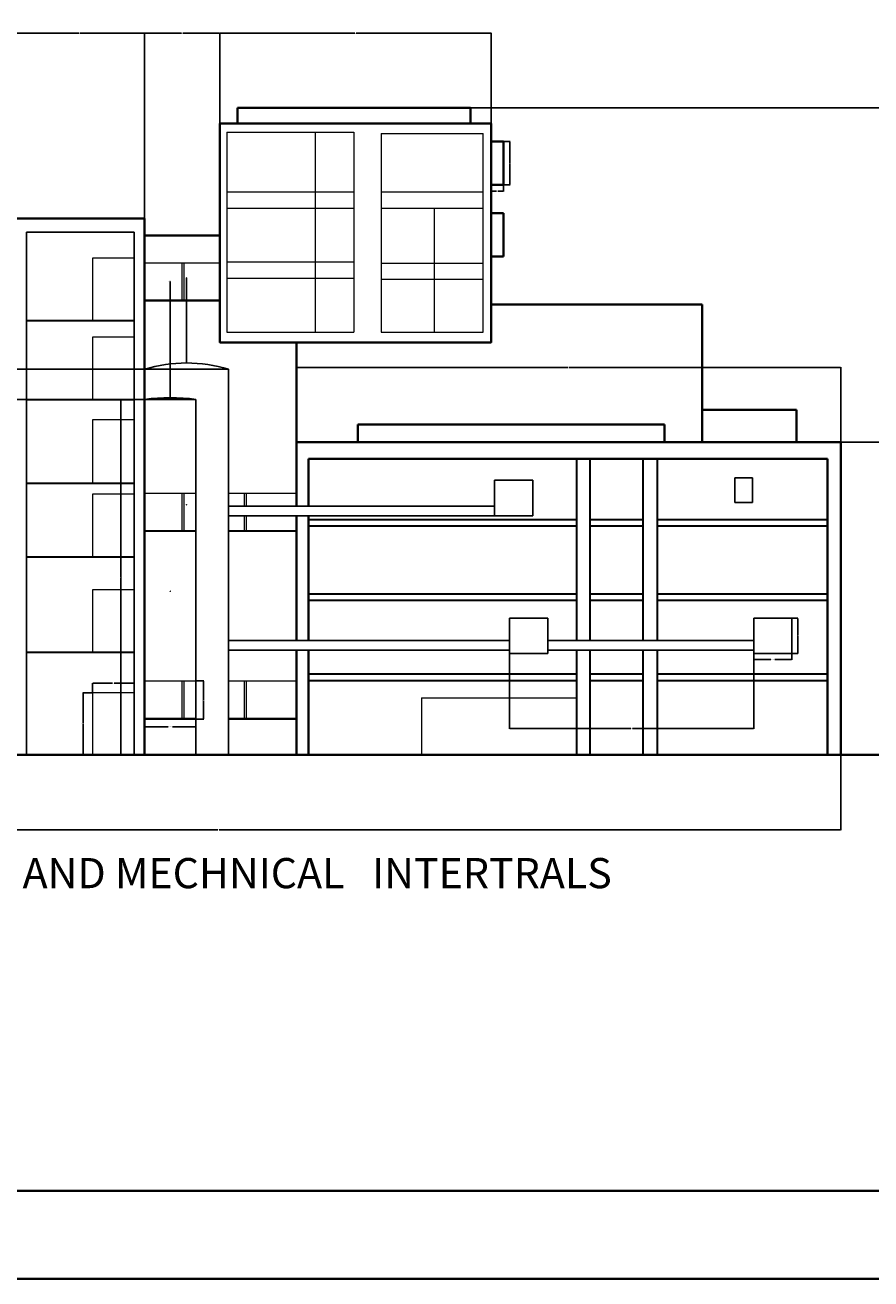
# Model space of a CAD drawing. Units: inches. Extents: x -934 to 898, y -1502 to 444.
# Tile 3 of 10: x -246 to 268, y -1502 to -739. Entities that reach past the tile are written whole.
import ezdxf

# ---------------------------------------------------------------- set-up
doc = ezdxf.new("R2010")
doc.units = ezdxf.units.IN
doc.header["$MEASUREMENT"] = 0
for name, color, linetype, lineweight in [('A-ANNO-DIMS', 2, 'Continuous', 18), ('A-ANNO-TITL', 7, 'Continuous', 30), ('A-ANNO-TTLB', 7, 'Continuous', 35), ('A-COLS', 1, 'Continuous', 30), ('A-DOOR', 3, 'Continuous', 18), ('A-ELEV', 7, 'Continuous', 35), ('A-FLOR', 7, 'Continuous', 30), ('A-GLAZ', 4, 'Continuous', 13), ('A-ROOF', 7, 'Continuous', 35), ('L-GRND', 7, 'Continuous', 35), ('M-HVAC', 6, 'Continuous', 25)]:
    doc.layers.add(name, color=color, linetype=linetype, lineweight=lineweight)
doc.styles.get("Standard").update_dxf_attribs({"font": 'arial.ttf'})
doc.dimstyles.get("Standard").update_dxf_attribs({"dimtxt": 0.18, "dimasz": 0.18, "dimexe": 0.18, "dimexo": 0.0625, "dimgap": 0.09, "dimtad": 0, "dimtih": 1, "dimtoh": 1, "dimdec": 4, "dimzin": 0, "dimdsep": 46, "dimtxsty": 'Standard', "dimcen": 0.09, "dimadec": 0, "dimazin": 0, "dimtfac": 1, "dimtdec": 4, "dimtofl": 0, "dimtmove": 0, "dimatfit": 3, "dimfxl": 1, "dimtolj": 1, "dimtzin": 0, "dimarcsym": 0})

# ---------------------------------------------------------------- blocks, each defined once
blk = doc.blocks.new('CORE-ACCESS-OPENING')
for p, q in [((25.27, 37.91), (0, 37.91)), ((0, 37.91), (0, 0))]:
    blk.add_line(p, q)
blk = doc.blocks.new('FACADE-PROJECTION-SHORT')
for p, q in [((0, 26.24), (7.46, 26.24)), ((7.46, 26.24), (7.46, 0)), ((7.46, 0), (0, 0))]:
    blk.add_line(p, q)
blk = doc.blocks.new('MECH-TERMINAL')
for p, q in [((0, 15.62), (0, 21.53)), ((0, 21.53), (23.24, 21.53)), ((0, 15.62), (0, 21.53)), ((0, 21.53), (23.24, 21.53)), ((0, 0), (0, 15.62)), ((0, 0), (0, 15.62)), ((23.24, 21.53), (23.24, 0)), ((23.24, 21.53), (23.24, 0)), ((23.24, 0), (0, 0)), ((23.24, 0), (0, 0))]:
    blk.add_line(p, q)
blk = doc.blocks.new('SHAFT-CONNECTOR-BAY')
for p, q in [((0, 23.2), (31.08, 23.2)), ((22.68, 23.2), (22.68, 0)), ((23.92, 23.2), (23.92, 0)), ((0, 0.56), (31.08, 0.56)), ((23.92, 0.56), (31.08, 0.56)), ((0, 0), (31.08, 0)), ((23.92, 0), (31.08, 0))]:
    blk.add_line(p, q)
blk = doc.blocks.new('*D67')
at = {"layer": 'A-ANNO-DIMS', "color": 0, "lineweight": -2, "transparency": 16777216}
for p, q in [((-204.98, -1145.23), (-210.79, -1145.23)), ((-210.61, -1145.41), (-210.61, -1164)), ((-210.61, -1182.96), (-210.61, -1164.37)), ((-204.98, -1183.14), (-210.79, -1183.14))]:
    blk.add_line(p, q, dxfattribs=at)
at = {"layer": 'A-ANNO-DIMS', "color": 0, "transparency": 16777216}
for points in [[(-210.64, -1145.41), (-210.58, -1145.41), (-210.61, -1145.23)], [(-210.64, -1182.96), (-210.58, -1182.96), (-210.61, -1183.14)]]:
    blk.add_solid(points, dxfattribs=at)
at = {"layer": 'Defpoints', "color": 0, "transparency": 16777216}
for p in [(-210.61, -1145.23), (-204.92, -1145.23), (-204.92, -1183.14)]:
    blk.add_point(p, dxfattribs=at)
at = {"layer": 'A-ANNO-DIMS', "color": 0, "transparency": 16777216, "insert": (-210.61, -1164.18), "char_height": 0.18, "attachment_point": 5}
blk.add_mtext('\\A1;ACCESS 38 TYP.', dxfattribs=at)
blk = doc.blocks.new('*D68')
at = {"layer": 'A-ANNO-DIMS', "color": 0, "lineweight": -2, "transparency": 16777216}
for p, q in [((-204.92, -1145.17), (-204.92, -1139.36)), ((-204.74, -1139.54), (-192.82, -1139.54)), ((-179.83, -1139.54), (-191.76, -1139.54)), ((-179.65, -1145.17), (-179.65, -1139.36))]:
    blk.add_line(p, q, dxfattribs=at)
at = {"layer": 'A-ANNO-DIMS', "color": 0, "transparency": 16777216}
for points in [[(-204.74, -1139.51), (-204.74, -1139.57), (-204.92, -1139.54)], [(-179.83, -1139.51), (-179.83, -1139.57), (-179.65, -1139.54)]]:
    blk.add_solid(points, dxfattribs=at)
at = {"layer": 'Defpoints', "color": 0, "transparency": 16777216}
for p in [(-179.65, -1139.54), (-204.92, -1145.23), (-179.65, -1145.23)]:
    blk.add_point(p, dxfattribs=at)
at = {"layer": 'A-ANNO-DIMS', "color": 0, "transparency": 16777216, "insert": (-192.29, -1139.54), "char_height": 0.18, "attachment_point": 5}
blk.add_mtext('\\A1;25 TYP.', dxfattribs=at)
blk = doc.blocks.new('*D73')
at = {"layer": 'A-ANNO-DIMS', "color": 0, "lineweight": -2, "transparency": 16777216}
for p, q in [((44.87, -810.22), (48.92, -810.22)), ((48.74, -810.4), (48.74, -823.16)), ((48.74, -836.28), (48.74, -823.53)), ((44.87, -836.46), (48.92, -836.46))]:
    blk.add_line(p, q, dxfattribs=at)
at = {"layer": 'A-ANNO-DIMS', "color": 0, "transparency": 16777216}
for points in [[(48.71, -810.4), (48.77, -810.4), (48.74, -810.22)], [(48.71, -836.28), (48.77, -836.28), (48.74, -836.46)]]:
    blk.add_solid(points, dxfattribs=at)
at = {"layer": 'Defpoints', "color": 0, "transparency": 16777216}
for p in [(44.81, -810.22), (48.74, -810.22), (44.81, -836.46)]:
    blk.add_point(p, dxfattribs=at)
at = {"layer": 'A-ANNO-DIMS', "color": 0, "transparency": 16777216, "insert": (48.74, -823.34), "char_height": 0.18, "attachment_point": 5}
blk.add_mtext('\\A1;POD FIN 26 TYP.', dxfattribs=at)
blk = doc.blocks.new('*D74')
at = {"layer": 'A-ANNO-DIMS', "color": 0, "lineweight": -2, "transparency": 16777216}
for p, q in [((37.35, -836.52), (37.35, -840.58)), ((44.81, -836.52), (44.81, -840.58)), ((37.53, -840.4), (40.62, -840.4)), ((44.63, -840.4), (41.54, -840.4))]:
    blk.add_line(p, q, dxfattribs=at)
at = {"layer": 'A-ANNO-DIMS', "color": 0, "transparency": 16777216}
for points in [[(37.53, -840.37), (37.53, -840.43), (37.35, -840.4)], [(44.63, -840.37), (44.63, -840.43), (44.81, -840.4)]]:
    blk.add_solid(points, dxfattribs=at)
at = {"layer": 'Defpoints', "color": 0, "transparency": 16777216}
for p in [(37.35, -836.46), (44.81, -836.46), (44.81, -840.4)]:
    blk.add_point(p, dxfattribs=at)
at = {"layer": 'A-ANNO-DIMS', "color": 0, "transparency": 16777216, "insert": (41.08, -840.4), "char_height": 0.18, "attachment_point": 5}
blk.add_mtext('\\A1;7 TYP.', dxfattribs=at)
blk = doc.blocks.new('*D75')
at = {"layer": 'A-ANNO-DIMS', "color": 0, "lineweight": -2, "transparency": 16777216}
for p, q in [((197.03, -1121.56), (197.03, -1125.17)), ((197.21, -1124.99), (207.45, -1124.99)), ((220.1, -1124.99), (209.85, -1124.99)), ((220.28, -1121.56), (220.28, -1125.17))]:
    blk.add_line(p, q, dxfattribs=at)
at = {"layer": 'A-ANNO-DIMS', "color": 0, "transparency": 16777216}
for points in [[(197.21, -1124.96), (197.21, -1125.02), (197.03, -1124.99)], [(220.1, -1124.96), (220.1, -1125.02), (220.28, -1124.99)]]:
    blk.add_solid(points, dxfattribs=at)
at = {"layer": 'Defpoints', "color": 0, "transparency": 16777216}
for p in [(197.03, -1121.5), (220.28, -1121.5), (220.28, -1124.99)]:
    blk.add_point(p, dxfattribs=at)
at = {"layer": 'A-ANNO-DIMS', "color": 0, "transparency": 16777216, "insert": (208.65, -1124.99), "char_height": 0.18, "attachment_point": 5}
blk.add_mtext('\\A1;TERMINAL 23 TYP.', dxfattribs=at)
blk = doc.blocks.new('*D76')
at = {"layer": 'A-ANNO-DIMS', "color": 0, "lineweight": -2, "transparency": 16777216}
for p, q in [((220.34, -1099.97), (223.94, -1099.97)), ((223.76, -1100.15), (223.76, -1110.55)), ((223.76, -1121.32), (223.76, -1110.92)), ((220.34, -1121.5), (223.94, -1121.5))]:
    blk.add_line(p, q, dxfattribs=at)
at = {"layer": 'A-ANNO-DIMS', "color": 0, "transparency": 16777216}
for points in [[(223.73, -1100.15), (223.79, -1100.15), (223.76, -1099.97)], [(223.73, -1121.32), (223.79, -1121.32), (223.76, -1121.5)]]:
    blk.add_solid(points, dxfattribs=at)
at = {"layer": 'Defpoints', "color": 0, "transparency": 16777216}
for p in [(220.28, -1099.97), (223.76, -1099.97), (220.28, -1121.5)]:
    blk.add_point(p, dxfattribs=at)
at = {"layer": 'A-ANNO-DIMS', "color": 0, "transparency": 16777216, "insert": (223.76, -1110.74), "char_height": 0.18, "attachment_point": 5}
blk.add_mtext('\\A1;22 TYP.', dxfattribs=at)
blk = doc.blocks.new('*D77')
at = {"layer": 'A-ANNO-DIMS', "color": 0, "lineweight": -2, "transparency": 16777216}
for p, q in [((-173.27, -1161.38), (-173.27, -1166.16)), ((-173.09, -1165.98), (-159.02, -1165.98)), ((-142.37, -1165.98), (-156.44, -1165.98)), ((-142.19, -1161.38), (-142.19, -1166.16))]:
    blk.add_line(p, q, dxfattribs=at)
at = {"layer": 'A-ANNO-DIMS', "color": 0, "transparency": 16777216}
for points in [[(-173.09, -1165.95), (-173.09, -1166.01), (-173.27, -1165.98)], [(-142.37, -1165.95), (-142.37, -1166.01), (-142.19, -1165.98)]]:
    blk.add_solid(points, dxfattribs=at)
at = {"layer": 'Defpoints', "color": 0, "transparency": 16777216}
for p in [(-173.27, -1161.32), (-142.19, -1161.32), (-142.19, -1165.98)]:
    blk.add_point(p, dxfattribs=at)
at = {"layer": 'A-ANNO-DIMS', "color": 0, "transparency": 16777216, "insert": (-157.73, -1165.98), "char_height": 0.18, "attachment_point": 5}
blk.add_mtext('\\A1;SHAFT LINK 31 TYP.', dxfattribs=at)
blk = doc.blocks.new('*D78')
at = {"layer": 'A-ANNO-DIMS', "color": 0, "lineweight": -2, "transparency": 16777216}
for p, q in [((-142.13, -1138.12), (-137.35, -1138.12)), ((-137.53, -1138.3), (-137.53, -1149.54)), ((-137.53, -1161.14), (-137.53, -1149.9)), ((-142.13, -1161.32), (-137.35, -1161.32))]:
    blk.add_line(p, q, dxfattribs=at)
at = {"layer": 'A-ANNO-DIMS', "color": 0, "transparency": 16777216}
for points in [[(-137.56, -1138.3), (-137.5, -1138.3), (-137.53, -1138.12)], [(-137.56, -1161.14), (-137.5, -1161.14), (-137.53, -1161.32)]]:
    blk.add_solid(points, dxfattribs=at)
at = {"layer": 'Defpoints', "color": 0, "transparency": 16777216}
for p in [(-142.19, -1138.12), (-137.53, -1138.12), (-142.19, -1161.32)]:
    blk.add_point(p, dxfattribs=at)
at = {"layer": 'A-ANNO-DIMS', "color": 0, "transparency": 16777216, "insert": (-137.53, -1149.72), "char_height": 0.18, "attachment_point": 5}
blk.add_mtext('\\A1;23 TYP.', dxfattribs=at)
blk = doc.blocks.new('*D107')
at = {"layer": 'A-ANNO-DIMS', "color": 0, "lineweight": -2, "transparency": 16777216}
for p, q in [((-506.87, -1056.49), (-506.87, -1228.82)), ((249.98, -1183.07), (249.98, -1228.82)), ((-506.69, -1228.64), (-128.84, -1228.64)), ((249.8, -1228.64), (-128.05, -1228.64))]:
    blk.add_line(p, q, dxfattribs=at)
at = {"layer": 'A-ANNO-DIMS', "color": 0, "transparency": 16777216}
for points in [[(-506.69, -1228.61), (-506.69, -1228.67), (-506.87, -1228.64)], [(249.8, -1228.61), (249.8, -1228.67), (249.98, -1228.64)]]:
    blk.add_solid(points, dxfattribs=at)
at = {"layer": 'Defpoints', "color": 0, "transparency": 16777216}
for p in [(-506.87, -1056.43), (249.98, -1183.01), (249.98, -1228.64)]:
    blk.add_point(p, dxfattribs=at)
at = {"layer": 'A-ANNO-DIMS', "color": 0, "transparency": 16777216, "insert": (-128.45, -1228.64), "char_height": 0.18, "attachment_point": 5}
blk.add_mtext('\\A1;756.8', dxfattribs=at)
blk = doc.blocks.new('*D108')
at = {"layer": 'A-ANNO-DIMS', "color": 0, "lineweight": -2, "transparency": 16777216}
for p, q in [((24.87, -789.83), (353.87, -789.83)), ((353.69, -790.01), (353.69, -986.24)), ((353.69, -1182.83), (353.69, -986.6)), ((250.04, -1183.01), (353.87, -1183.01))]:
    blk.add_line(p, q, dxfattribs=at)
at = {"layer": 'A-ANNO-DIMS', "color": 0, "transparency": 16777216}
for points in [[(353.66, -790.01), (353.72, -790.01), (353.69, -789.83)], [(353.66, -1182.83), (353.72, -1182.83), (353.69, -1183.01)]]:
    blk.add_solid(points, dxfattribs=at)
at = {"layer": 'Defpoints', "color": 0, "transparency": 16777216}
for p in [(24.8, -789.83), (353.69, -789.83), (249.98, -1183.01)]:
    blk.add_point(p, dxfattribs=at)
at = {"layer": 'A-ANNO-DIMS', "color": 0, "transparency": 16777216, "insert": (353.69, -986.42), "char_height": 0.18, "attachment_point": 5}
blk.add_mtext('\\A1;393.2', dxfattribs=at)
blk = doc.blocks.new('*D110')
at = {"layer": 'A-ANNO-DIMS', "color": 0, "lineweight": -2, "transparency": 16777216}
for p, q in [((-252.7, -856.85), (-252.7, -744.15)), ((-252.52, -744.33), (-213.38, -744.33)), ((-173.45, -744.33), (-212.59, -744.33)), ((-173.27, -856.85), (-173.27, -744.15))]:
    blk.add_line(p, q, dxfattribs=at)
at = {"layer": 'A-ANNO-DIMS', "color": 0, "transparency": 16777216}
for points in [[(-252.52, -744.3), (-252.52, -744.36), (-252.7, -744.33)], [(-173.45, -744.3), (-173.45, -744.36), (-173.27, -744.33)]]:
    blk.add_solid(points, dxfattribs=at)
at = {"layer": 'Defpoints', "color": 0, "transparency": 16777216}
for p in [(-173.27, -744.33), (-252.7, -856.91), (-173.27, -856.91)]:
    blk.add_point(p, dxfattribs=at)
at = {"layer": 'A-ANNO-DIMS', "color": 0, "transparency": 16777216, "insert": (-212.98, -744.33), "char_height": 0.18, "attachment_point": 5}
blk.add_mtext('\\A1;79.43', dxfattribs=at)
blk = doc.blocks.new('*D111')
at = {"layer": 'A-ANNO-DIMS', "color": 0, "lineweight": -2, "transparency": 16777216}
for p, q in [((-127.51, -799.26), (-127.51, -744.15)), ((-127.33, -744.33), (-45.54, -744.33)), ((37.17, -744.33), (-44.62, -744.33)), ((37.35, -799.26), (37.35, -744.15))]:
    blk.add_line(p, q, dxfattribs=at)
at = {"layer": 'A-ANNO-DIMS', "color": 0, "transparency": 16777216}
for points in [[(-127.33, -744.3), (-127.33, -744.36), (-127.51, -744.33)], [(37.17, -744.3), (37.17, -744.36), (37.35, -744.33)]]:
    blk.add_solid(points, dxfattribs=at)
at = {"layer": 'Defpoints', "color": 0, "transparency": 16777216}
for p in [(37.35, -744.33), (-127.51, -799.32), (37.35, -799.32)]:
    blk.add_point(p, dxfattribs=at)
at = {"layer": 'A-ANNO-DIMS', "color": 0, "transparency": 16777216, "insert": (-45.08, -744.33), "char_height": 0.18, "attachment_point": 5}
blk.add_mtext('\\A1;164.85', dxfattribs=at)
blk = doc.blocks.new('*D112')
at = {"layer": 'A-ANNO-DIMS', "color": 0, "lineweight": -2, "transparency": 16777216}
for p, q in [((-80.93, -992.98), (-80.93, -947.36)), ((-80.75, -947.54), (84.13, -947.54)), ((249.8, -947.54), (84.92, -947.54)), ((249.98, -992.98), (249.98, -947.36))]:
    blk.add_line(p, q, dxfattribs=at)
at = {"layer": 'A-ANNO-DIMS', "color": 0, "transparency": 16777216}
for points in [[(-80.75, -947.51), (-80.75, -947.57), (-80.93, -947.54)], [(249.8, -947.51), (249.8, -947.57), (249.98, -947.54)]]:
    blk.add_solid(points, dxfattribs=at)
at = {"layer": 'Defpoints', "color": 0, "transparency": 16777216}
for p in [(249.98, -947.54), (-80.93, -993.04), (249.98, -993.04)]:
    blk.add_point(p, dxfattribs=at)
at = {"layer": 'A-ANNO-DIMS', "color": 0, "transparency": 16777216, "insert": (84.52, -947.54), "char_height": 0.18, "attachment_point": 5}
blk.add_mtext('\\A1;330.9', dxfattribs=at)
blk = doc.blocks.new('*D113')
at = {"layer": 'A-ANNO-DIMS', "color": 0, "lineweight": -2, "transparency": 16777216}
for p, q in [((250.04, -993.04), (295.66, -993.04)), ((295.48, -993.22), (295.48, -1087.84)), ((295.48, -1182.83), (295.48, -1088.21)), ((250.04, -1183.01), (295.66, -1183.01))]:
    blk.add_line(p, q, dxfattribs=at)
at = {"layer": 'A-ANNO-DIMS', "color": 0, "transparency": 16777216}
for points in [[(295.45, -993.22), (295.51, -993.22), (295.48, -993.04)], [(295.45, -1182.83), (295.51, -1182.83), (295.48, -1183.01)]]:
    blk.add_solid(points, dxfattribs=at)
at = {"layer": 'Defpoints', "color": 0, "transparency": 16777216}
for p in [(249.98, -993.04), (249.98, -1183.01), (295.48, -1183.01)]:
    blk.add_point(p, dxfattribs=at)
at = {"layer": 'A-ANNO-DIMS', "color": 0, "transparency": 16777216, "insert": (295.48, -1088.02), "char_height": 0.18, "attachment_point": 5}
blk.add_mtext('\\A1;189.97', dxfattribs=at)
blk = doc.blocks.new('*D114')
at = {"layer": 'A-ANNO-DIMS', "color": 0, "lineweight": -2, "transparency": 16777216}
for p, q in [((-122.37, -948.66), (-637.55, -948.66)), ((-637.37, -948.84), (-637.37, -957.63)), ((-637.37, -966.78), (-637.37, -957.99)), ((-142.26, -966.96), (-637.55, -966.96))]:
    blk.add_line(p, q, dxfattribs=at)
at = {"layer": 'A-ANNO-DIMS', "color": 0, "transparency": 16777216}
for points in [[(-637.4, -948.84), (-637.34, -948.84), (-637.37, -948.66)], [(-637.4, -966.78), (-637.34, -966.78), (-637.37, -966.96)]]:
    blk.add_solid(points, dxfattribs=at)
at = {"layer": 'Defpoints', "color": 0, "transparency": 16777216}
for p in [(-637.37, -948.66), (-122.31, -948.66), (-142.19, -966.96)]:
    blk.add_point(p, dxfattribs=at)
at = {"layer": 'A-ANNO-DIMS', "color": 0, "transparency": 16777216, "insert": (-637.37, -957.81), "char_height": 0.18, "attachment_point": 5}
blk.add_mtext('\\A1;18.294', dxfattribs=at)
blk = doc.blocks.new('*D115')
at = {"layer": 'A-ANNO-DIMS', "color": 0, "lineweight": -2, "transparency": 16777216}
for p, q in [((-142.26, -966.96), (-187.87, -966.96)), ((-187.69, -967.14), (-187.69, -1074.8)), ((-187.69, -1182.83), (-187.69, -1075.17)), ((-142.26, -1183.01), (-187.87, -1183.01))]:
    blk.add_line(p, q, dxfattribs=at)
at = {"layer": 'A-ANNO-DIMS', "color": 0, "transparency": 16777216}
for points in [[(-187.72, -967.14), (-187.66, -967.14), (-187.69, -966.96)], [(-187.72, -1182.83), (-187.66, -1182.83), (-187.69, -1183.01)]]:
    blk.add_solid(points, dxfattribs=at)
at = {"layer": 'Defpoints', "color": 0, "transparency": 16777216}
for p in [(-187.69, -966.96), (-142.19, -966.96), (-142.19, -1183.01)]:
    blk.add_point(p, dxfattribs=at)
at = {"layer": 'A-ANNO-DIMS', "color": 0, "transparency": 16777216, "insert": (-187.69, -1074.98), "char_height": 0.18, "attachment_point": 5}
blk.add_mtext('\\A1;216.05', dxfattribs=at)
blk = doc.blocks.new('*D116')
at = {"layer": 'A-ANNO-DIMS', "color": 0, "lineweight": -2, "transparency": 16777216}
for p, q in [((-173.27, -856.85), (-173.27, -744.15)), ((-173.09, -744.33), (-150.79, -744.33)), ((-127.69, -744.33), (-149.99, -744.33)), ((-127.51, -799.26), (-127.51, -744.15))]:
    blk.add_line(p, q, dxfattribs=at)
at = {"layer": 'A-ANNO-DIMS', "color": 0, "transparency": 16777216}
for points in [[(-173.09, -744.3), (-173.09, -744.36), (-173.27, -744.33)], [(-127.69, -744.3), (-127.69, -744.36), (-127.51, -744.33)]]:
    blk.add_solid(points, dxfattribs=at)
at = {"layer": 'Defpoints', "color": 0, "transparency": 16777216}
for p in [(-127.51, -744.33), (-127.51, -799.32), (-173.27, -856.91)]:
    blk.add_point(p, dxfattribs=at)
at = {"layer": 'A-ANNO-DIMS', "color": 0, "transparency": 16777216, "insert": (-150.39, -744.33), "char_height": 0.18, "attachment_point": 5}
blk.add_mtext('\\A1;45.76', dxfattribs=at)
blk = doc.blocks.new('*D118')
at = {"layer": 'A-ANNO-DIMS', "color": 0, "lineweight": -2, "transparency": 16777216}
for p, q in [((48.56, -1121.56), (48.56, -1167.18)), ((197.03, -1121.56), (197.03, -1167.18)), ((48.74, -1167), (122.34, -1167)), ((196.85, -1167), (123.25, -1167))]:
    blk.add_line(p, q, dxfattribs=at)
at = {"layer": 'A-ANNO-DIMS', "color": 0, "transparency": 16777216}
for points in [[(48.74, -1166.97), (48.74, -1167.03), (48.56, -1167)], [(196.85, -1166.97), (196.85, -1167.03), (197.03, -1167)]]:
    blk.add_solid(points, dxfattribs=at)
at = {"layer": 'Defpoints', "color": 0, "transparency": 16777216}
for p in [(48.56, -1121.5), (197.03, -1121.5), (48.56, -1167)]:
    blk.add_point(p, dxfattribs=at)
at = {"layer": 'A-ANNO-DIMS', "color": 0, "transparency": 16777216, "insert": (122.79, -1167), "char_height": 0.18, "attachment_point": 5}
blk.add_mtext('\\A1;148.48', dxfattribs=at)
blk = doc.blocks.new('*D119')
at = {"layer": 'A-ANNO-DIMS', "color": 0, "lineweight": -2, "transparency": 16777216}
for p, q in [((-147.99, -893.1), (-147.81, -893.1)), ((-147.81, -893.1), (-147.8, -944.63)), ((-147.88, -1031), (-147.7, -1031)), ((-147.79, -1031.09), (-147.79, -1030.91))]:
    blk.add_line(p, q, dxfattribs=at)
at = {"layer": 'A-ANNO-DIMS', "color": 0, "transparency": 16777216}
blk.add_solid([(-147.77, -944.63), (-147.83, -944.63), (-147.8, -944.81)], dxfattribs=at)
at = {"layer": 'Defpoints', "color": 0, "transparency": 16777216}
for p in [(-147.8, -944.81), (-147.79, -1031)]:
    blk.add_point(p, dxfattribs=at)
at = {"layer": 'A-ANNO-DIMS', "color": 0, "transparency": 16777216, "insert": (-148.47, -893.1), "char_height": 0.18, "attachment_point": 5}
blk.add_mtext('\\A1;R86.19', dxfattribs=at)
blk = doc.blocks.new('*D120')
at = {"layer": 'A-ANNO-DIMS', "color": 0, "lineweight": -2, "transparency": 16777216}
for p, q in [((-158.02, -895.36), (-157.84, -895.36)), ((-157.84, -895.36), (-157.8, -965.75)), ((-157.82, -1083.54), (-157.64, -1083.54)), ((-157.73, -1083.63), (-157.73, -1083.45))]:
    blk.add_line(p, q, dxfattribs=at)
at = {"layer": 'A-ANNO-DIMS', "color": 0, "transparency": 16777216}
blk.add_solid([(-157.77, -965.75), (-157.83, -965.75), (-157.8, -965.93)], dxfattribs=at)
at = {"layer": 'Defpoints', "color": 0, "transparency": 16777216}
for p in [(-157.8, -965.93), (-157.73, -1083.54)]:
    blk.add_point(p, dxfattribs=at)
at = {"layer": 'A-ANNO-DIMS', "color": 0, "transparency": 16777216, "insert": (-158.5, -895.36), "char_height": 0.18, "attachment_point": 5}
blk.add_mtext('\\A1;R117.6', dxfattribs=at)

msp = doc.modelspace()

# ---------------------------------------------------------------- linework, layer by layer
at = {"layer": 'A-ANNO-TTLB'}
for points in [[(-933.5092, 444.4646), (897.7239, 444.4646), (897.7239, -1501.5858), (-933.5092, -1501.5858)], [(-892.081, 380.0228), (832.9871, 380.0228), (832.9871, -1448.0237), (-892.081, -1448.0237)]]:
    msp.add_lwpolyline(points, close=True, dxfattribs=at)
at = {"layer": 'A-COLS'}
for p, q in [((89.3499, -1003.181), (89.3499, -1113.4354)), ((97.3121, -1003.181), (97.3121, -1113.4354)), ((129.8979, -1113.4354), (129.8979, -1003.181)), ((138.3057, -1003.181), (138.3057, -1113.4354)), ((89.3499, -1119.4824), (89.3499, -1183.0104)), ((97.3121, -1119.4824), (97.3121, -1183.0104)), ((129.8979, -1183.0104), (129.8979, -1119.4824)), ((138.3057, -1119.4824), (138.3057, -1183.0104))]:
    msp.add_line(p, q, dxfattribs=at)
at = {"layer": 'A-DOOR'}
for q in [(-4.8589, -1183.0104), (89.3499, -1148.339)]:
    msp.add_line((-4.8589, -1148.339), q, dxfattribs=at)
at = {"layer": 'A-ELEV'}
for p, q in [((-173.2689, -856.9131), (-252.6991, -856.9131)), ((-173.2689, -867.3393), (-173.2689, -856.9131)), ((-173.2689, -867.3393), (-149.994, -867.3393)), ((-173.2689, -867.3393), (-173.2689, -1183.0104)), ((-127.5081, -867.3393), (-149.994, -867.3393)), ((37.3466, -909.3175), (165.6865, -909.3175)), ((165.6865, -909.3175), (165.6865, -993.0377)), ((-80.9314, -993.0377), (-80.9314, -932.2941)), ((165.6865, -973.27), (223.0548, -973.27)), ((223.0548, -973.27), (223.0548, -993.0377)), ((165.6865, -993.0377), (-80.9314, -993.0377)), ((-80.9314, -993.0377), (-80.9314, -1031.9101)), ((165.6865, -993.0377), (249.977, -993.0377)), ((249.977, -993.0377), (249.977, -1183.0104)), ((138.3057, -1003.181), (-73.6255, -1003.181)), ((-73.6255, -1031.9101), (-73.6255, -1003.181)), ((241.7923, -1003.181), (138.3057, -1003.181)), ((241.7923, -1183.0104), (241.7923, -1003.181)), ((-80.9314, -1037.6812), (-80.9314, -1113.4354)), ((-73.6255, -1113.4354), (-73.6255, -1037.6812)), ((-80.9314, -1119.4824), (-80.9314, -1183.0104)), ((-73.6255, -1183.0104), (-73.6255, -1119.4824))]:
    msp.add_line(p, q, dxfattribs=at)
msp.add_lwpolyline([(-127.5081, -799.323), (37.3466, -799.323), (37.3466, -932.2941), (-127.5081, -932.2941)], close=True, dxfattribs=at)
at = {"layer": 'A-FLOR'}
for p, q in [((-245.0847, -919.0154), (-179.6533, -919.0154)), ((-245.0847, -966.9581), (-179.6533, -966.9581)), ((-245.0847, -1017.8497), (-179.6533, -1017.8497)), ((-73.6255, -1039.9197), (89.3499, -1039.9197)), ((-73.6255, -1043.9149), (89.3499, -1043.9149)), ((97.3121, -1039.9197), (129.8979, -1039.9197)), ((97.3121, -1043.9149), (129.8979, -1043.9149)), ((138.3057, -1039.9197), (241.7923, -1039.9197)), ((138.3057, -1043.9149), (241.7923, -1043.9149)), ((-245.0847, -1062.7319), (-179.6533, -1062.7319)), ((-73.6255, -1085.0557), (89.3499, -1085.0557)), ((-73.6255, -1089.0509), (89.3499, -1089.0509)), ((97.3121, -1085.0557), (129.8979, -1085.0557)), ((97.3121, -1089.0509), (129.8979, -1089.0509)), ((138.3057, -1085.0557), (241.7923, -1085.0557)), ((138.3057, -1089.0509), (241.7923, -1089.0509)), ((-245.0847, -1120.603), (-179.6533, -1120.603)), ((-73.6255, -1133.7514), (89.3499, -1133.7514)), ((97.3121, -1133.7514), (129.8979, -1133.7514)), ((138.3057, -1133.7514), (241.7923, -1133.7514)), ((-73.6255, -1137.7467), (89.3499, -1137.7467)), ((97.3121, -1137.7467), (129.8979, -1137.7467)), ((138.3057, -1137.7467), (241.7923, -1137.7467))]:
    msp.add_line(p, q, dxfattribs=at)
at = {"layer": 'A-GLAZ'}
for p, q in [((-123.3989, -804.4452), (-123.3989, -926.1337)), ((-123.3989, -804.4452), (-46.0534, -804.4452)), ((-69.6934, -804.4452), (-69.6934, -926.1337)), ((-46.0534, -804.4452), (-46.0534, -926.1337)), ((-29.5446, -805.3973), (-29.5446, -926.1337)), ((-29.5446, -805.3973), (32.5945, -805.3973)), ((32.5945, -926.1337), (32.5945, -805.3973)), ((-123.3989, -840.8503), (-46.0534, -840.8503)), ((-29.5446, -840.8503), (32.5945, -840.8503)), ((-46.0534, -850.9555), (-123.3989, -850.9555)), ((32.5945, -850.9555), (-29.5446, -850.9555)), ((2.6953, -850.9555), (2.6953, -926.1337)), ((-173.2689, -883.8841), (-127.5081, -883.8841)), ((-150.5913, -883.8841), (-150.5913, -907.0873)), ((-149.3497, -883.8841), (-149.3497, -907.0873)), ((-123.3989, -883.3385), (-46.0534, -883.3385)), ((-29.5446, -884.0631), (32.5945, -884.0631)), ((-46.0534, -893.4437), (-123.3989, -893.4437)), ((32.5945, -894.1684), (-29.5446, -894.1684)), ((-173.2689, -906.532), (-127.5081, -906.532)), ((-173.2689, -907.0873), (-127.5081, -907.0873)), ((-123.3989, -926.1337), (-46.0534, -926.1337)), ((-29.5446, -926.1337), (32.5945, -926.1337)), ((-122.305, -1023.9491), (-80.9314, -1023.9491)), ((-112.8003, -1023.9491), (-112.8003, -1031.9101)), ((-111.5587, -1023.9491), (-111.5587, -1031.9101)), ((-112.8003, -1037.6812), (-112.8003, -1047.1524)), ((-111.5587, -1037.6812), (-111.5587, -1047.1524)), ((-122.305, -1046.597), (-80.9314, -1046.597)), ((-122.305, -1047.1524), (-80.9314, -1047.1524)), ((-122.305, -1138.1178), (-80.9314, -1138.1178)), ((-112.8003, -1138.1178), (-112.8003, -1161.321)), ((-111.5587, -1138.1178), (-111.5587, -1161.321)), ((-122.305, -1160.7656), (-80.9314, -1160.7656)), ((-122.305, -1161.321), (-80.9314, -1161.321))]:
    msp.add_line(p, q, dxfattribs=at)
at = {"layer": 'A-ROOF'}
for p, q in [((-116.8608, -799.323), (-116.8608, -789.826)), ((-116.8608, -789.826), (24.8027, -789.826)), ((24.8027, -789.826), (24.8027, -799.323)), ((-43.5956, -993.0377), (-43.5956, -982.2041)), ((-43.5956, -982.2041), (142.7729, -982.2041)), ((142.7729, -982.2041), (142.7729, -993.0377))]:
    msp.add_line(p, q, dxfattribs=at)
at = {"layer": 'L-GRND'}
msp.add_line((-288.9776, -1183.0104), (308.1933, -1183.0104), dxfattribs=at)
at = {"layer": 'M-HVAC'}
for p, q in [((-245.0847, -865.3807), (-179.6533, -865.3807)), ((-245.0847, -865.3807), (-245.0847, -1183.0104)), ((-179.6533, -865.3807), (-179.6533, -1183.0104)), ((-122.305, -948.6643), (-122.305, -1183.0104)), ((-142.1926, -966.9581), (-142.1926, -1183.0104)), ((185.5343, -1014.7389), (185.5343, -1029.7276)), ((196.3286, -1014.7389), (185.5343, -1014.7389)), ((196.3286, -1029.7276), (196.3286, -1014.7389)), ((-122.305, -1031.9101), (39.499, -1031.9101)), ((185.5343, -1029.7276), (196.3286, -1029.7276)), ((39.499, -1037.6812), (-122.305, -1037.6812)), ((48.5552, -1113.4354), (-122.305, -1113.4354)), ((48.5552, -1119.4824), (-122.305, -1119.4824)), ((197.031, -1113.4354), (71.8001, -1113.4354)), ((197.031, -1119.4824), (71.8001, -1119.4824))]:
    msp.add_line(p, q, dxfattribs=at)
for centre, radius, start, end in [((-147.787, -1030.9986), 86.1874, 72.8030571, 107.1969429), ((-157.7307, -1083.5388), 117.6116, 82.4082307, 97.5917693)]:
    msp.add_arc(centre, radius, start, end, dxfattribs=at)

# ---------------------------------------------------------------- block references
at = {"layer": 'A-DOOR'}
for p in [(-204.9217, -919.0154), (-204.9217, -966.9597), (-204.9217, -1017.3326), (-204.9217, -1062.4813), (-204.9217, -1120.5349), (-204.9217, -1183.1394)]:
    msp.add_blockref('CORE-ACCESS-OPENING', p, dxfattribs=at)
at = {"layer": 'A-ELEV'}
for p in [(37.3466, -836.4622), (37.3466, -880.0122)]:
    msp.add_blockref('FACADE-PROJECTION-SHORT', p, dxfattribs=at)
at = {"layer": 'A-GLAZ'}
for p in [(-173.2689, -1047.1524), (-173.2689, -1161.321)]:
    msp.add_blockref('SHAFT-CONNECTOR-BAY', p, dxfattribs=at)
at = {"layer": 'M-HVAC'}
for p in [(39.499, -1037.6812), (48.5552, -1121.4997), (197.031, -1121.4997)]:
    msp.add_blockref('MECH-TERMINAL', p, dxfattribs=at)

# ---------------------------------------------------------------- texts
at = {"layer": 'A-ANNO-TITL'}
msp.add_text('SIDE   ELEVATION   AND MECHNICAL   INTERTRALS', height=18.353224, dxfattribs=at).set_placement((-467.0954, -1264.0952))

# ---------------------------------------------------------------- dimensions: what is measured, and where the dimension line sits
at = {"layer": 'A-ANNO-DIMS'}
for base, p1, p2, override, picture, middle in [((-173.2689, -744.326), (-252.6991, -856.9131), (-173.2689, -856.9131), {"dimdec": 2, "dimlfac": 1, "dimrnd": 0, "dimzin": 0, "dimdsep": 46, "dimlunit": 2}, '*D110', (-212.984, -744.326)), ((-127.5081, -744.326), (-173.2689, -856.9131), (-127.5081, -799.323), {"dimdec": 2, "dimlfac": 1, "dimrnd": 0, "dimzin": 0, "dimdsep": 46, "dimlunit": 2}, '*D116', (-150.3885, -744.326)), ((37.3466, -744.326), (-127.5081, -799.323), (37.3466, -799.323), {"dimdec": 2, "dimlfac": 1, "dimrnd": 0, "dimzin": 0, "dimdsep": 46, "dimlunit": 2}, '*D111', (-45.0808, -744.326)), ((249.977, -947.5377), (-80.9314, -993.0377), (249.977, -993.0377), {"dimdec": 1, "dimlfac": 1, "dimrnd": 0, "dimzin": 0, "dimdsep": 46, "dimlunit": 2}, '*D112', (84.5228, -947.5377)), ((249.977, -1228.6394), (-506.8678, -1056.4266), (249.977, -1183.0104), {"dimdec": 1, "dimlfac": 1, "dimrnd": 0, "dimzin": 0, "dimdsep": 46, "dimlunit": 2}, '*D107', (-128.4454, -1228.6394))]:
    dim = msp.add_linear_dim(base=base, p1=p1, p2=p2, dimstyle='Standard', override=override, dxfattribs=at)
    dim.commit()
    dim.dimension.update_dxf_attribs({"geometry": picture, "text_midpoint": middle})
for base, p1, p2, angle, override, picture, middle in [((353.6933, -789.826), (249.977, -1183.0104), (24.8027, -789.826), 90, {"dimdec": 1, "dimlfac": 1, "dimrnd": 0, "dimzin": 0, "dimdsep": 46, "dimlunit": 2}, '*D108', (353.6933, -986.4182)), ((-637.3658, -948.6643), (-142.1926, -966.9581), (-122.305, -948.6643), 90, {"dimdec": 3, "dimlfac": 1, "dimrnd": 0, "dimzin": 0, "dimdsep": 46, "dimlunit": 2}, '*D114', (-637.3658, -957.8112)), ((-187.6926, -966.9581), (-142.1926, -1183.0104), (-142.1926, -966.9581), 90, {"dimdec": 2, "dimlfac": 1, "dimrnd": 0, "dimzin": 0, "dimdsep": 46, "dimlunit": 2}, '*D115', (-187.6926, -1074.9843)), ((295.477, -1183.0104), (249.977, -993.0377), (249.977, -1183.0104), 270, {"dimdec": 2, "dimlfac": 1, "dimrnd": 0, "dimzin": 0, "dimdsep": 46, "dimlunit": 2}, '*D113', (295.477, -1088.024)), ((48.5552, -1166.9997), (197.031, -1121.4997), (48.5552, -1121.4997), 180, {"dimdec": 2, "dimlfac": 1, "dimrnd": 0, "dimzin": 0, "dimdsep": 46, "dimlunit": 2}, '*D118', (122.7931, -1166.9997))]:
    dim = msp.add_linear_dim(base=base, p1=p1, p2=p2, angle=angle, dimstyle='Standard', override=override, dxfattribs=at)
    dim.commit()
    dim.dimension.update_dxf_attribs({"geometry": picture, "text_midpoint": middle})
for base, p1, p2, text, picture, middle in [((48.7449, -810.2243), (44.8092, -836.4622), (44.8092, -810.2243), 'POD FIN <> TYP.', '*D73', (48.7449, -823.3433)), ((223.7627, -1099.9711), (220.2759, -1121.4997), (220.2759, -1099.9711), '<> TYP.', '*D76', (223.7627, -1110.7354)), ((-137.5312, -1138.1178), (-142.1926, -1161.321), (-142.1926, -1138.1178), '<> TYP.', '*D78', (-137.5312, -1149.7194)), ((-210.6085, -1145.2276), (-204.9217, -1183.1394), (-204.9217, -1145.2276), 'ACCESS <> TYP.', '*D67', (-210.6085, -1164.1835))]:
    dim = msp.add_linear_dim(base=base, p1=p1, p2=p2, angle=90, text=text, dimstyle='Standard', override={"dimdec": 0, "dimlfac": 1, "dimrnd": 0, "dimzin": 0, "dimdsep": 46, "dimlunit": 2}, dxfattribs=at)
    dim.commit()
    dim.dimension.update_dxf_attribs({"geometry": picture, "text_midpoint": middle})
for base, p1, p2, text, picture, middle in [((44.8092, -840.3979), (37.3466, -836.4622), (44.8092, -836.4622), '<> TYP.', '*D74', (41.0779, -840.3979)), ((220.2759, -1124.9864), (197.031, -1121.4997), (220.2759, -1121.4997), 'TERMINAL <> TYP.', '*D75', (208.6535, -1124.9864)), ((-179.6533, -1139.5409), (-204.9217, -1145.2276), (-179.6533, -1145.2276), '<> TYP.', '*D68', (-192.2875, -1139.5409)), ((-142.1926, -1165.9824), (-173.2689, -1161.321), (-142.1926, -1161.321), 'SHAFT LINK <> TYP.', '*D77', (-157.7307, -1165.9824))]:
    dim = msp.add_linear_dim(base=base, p1=p1, p2=p2, text=text, dimstyle='Standard', override={"dimdec": 0, "dimlfac": 1, "dimrnd": 0, "dimzin": 0, "dimdsep": 46, "dimlunit": 2}, dxfattribs=at)
    dim.commit()
    dim.dimension.update_dxf_attribs({"geometry": picture, "text_midpoint": middle})
for center, mpoint, override, picture, middle in [((-157.7307, -1083.5388), (-157.8, -965.9272), {"dimdec": 1, "dimlfac": 1, "dimrnd": 0, "dimzin": 0, "dimdsep": 46, "dimlunit": 2}, '*D120', (-158.5013, -895.3602)), ((-147.787, -1030.9986), (-147.8, -944.8112), {"dimdec": 2, "dimlfac": 1, "dimrnd": 0, "dimzin": 0, "dimdsep": 46, "dimlunit": 2}, '*D119', (-148.4678, -893.0987))]:
    dim = msp.add_radius_dim(center=center, mpoint=mpoint, dimstyle='Standard', override=override, dxfattribs=at)
    dim.commit()
    dim.dimension.update_dxf_attribs({"geometry": picture, "text_midpoint": middle, "dimtype": 164})

doc.saveas('drawing.dxf')
